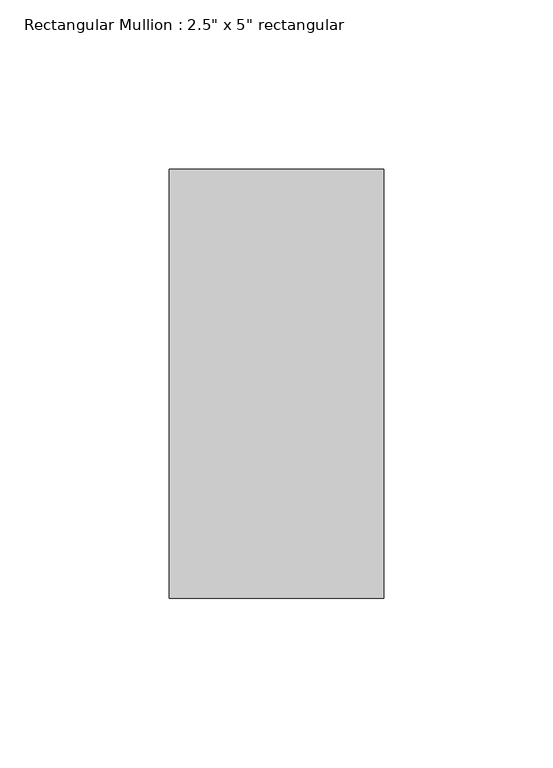
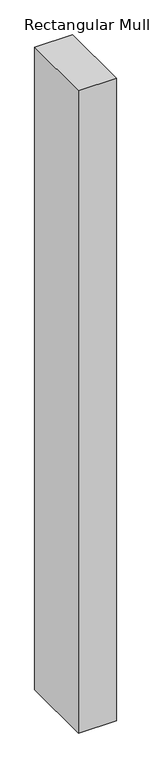
"""IFC4 building model written with IfcOpenShell, lengths in millimetres: member geometry."""

from ifc_helpers import new_model, si_unit, frame, origin, place, context, project, spatial, polyline, outline, extrude, source, transform, mapped, element, save


def member_64b232f9(model_context):
    return source(origin(), model_context, "Body", "SweptSolid", [
        extrude(outline(polyline([(31.75, 63.5), (31.75, -63.5), (-31.75, -63.5), (-31.75, 63.5), (31.75, 63.5)])), frame((0.0, 0.0, -1137.3648635), z_axis=(0.0, 0.0, 1.0), x_axis=(1.0, 0.0, 0.0)), (0.0, 0.0, 1.0), 1137.3648635),
    ])


if __name__ == "__main__":
    model = new_model("IFC4")
    model_context = context("Model", 3, world=origin())
    ifc_project = project(units=[si_unit("LENGTHUNIT", "METRE", prefix="MILLI")], contexts=[model_context])
    site = spatial("IfcSite", under=ifc_project)
    building = spatial("IfcBuilding", under=site)
    placement = place(None, origin())
    member_shape = member_64b232f9(model_context)
    element("IfcMember", 1, ObjectType="Rectangular Mullion : 2.5\" x 5\" rectangular", at=placement, inside=building, context=model_context, shape_type="MappedRepresentation", body=[
        mapped(member_shape, transform((0.0, 0.0, 0.0), x_axis=(1.0, 0.0, 0.0), y_axis=(0.0, 1.0, 0.0), z_axis=(0.0, 0.0, 1.0))),
    ])
    save(model, "model.ifc")

# Revit data of these elements
# Type "Rectangular Mullion : 2.5\" x 5\" rectangular"
#   built-in parameter 1007304 = 0.416667 (stored number, unit not read)
#   built-in parameter 1007301 = 0.104167 (stored number, unit not read)
#   built-in parameter 1007300 = 0.104167 (stored number, unit not read)
# Element 1 (IfcMember, "Rectangular Mullion : 2.5\" x 5\" rectangular")
#   Materials on its faces: "Aluminum"
# Materials
#   "Aluminum": class "Metal", colour RGB 247 247 247, transparency 0, Description = "Aluminum 6061", Cost = 0
